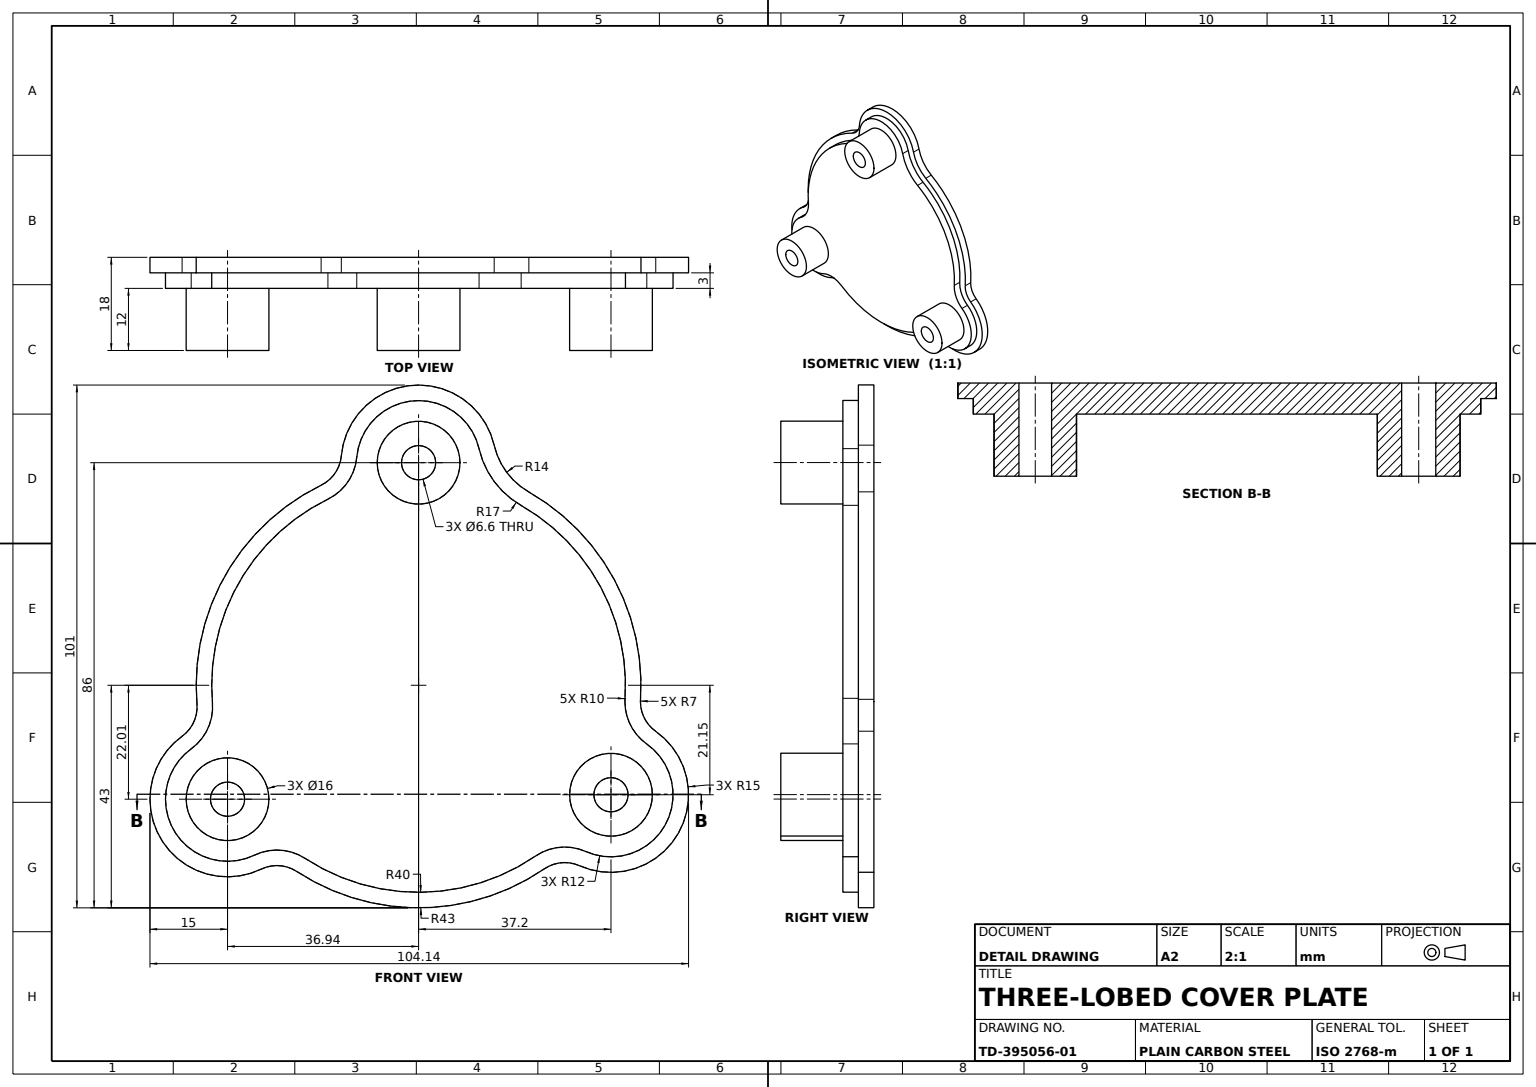
from build123d import *

# Parameters (mm, degrees)
BASE_PLATE_DEPTH               = 3
OFFSET_STEP_DEPTH              = 3
STANDOFF_BOSS_PROFILE_3X_16_R  = 8
STANDOFF_BOSSES_3X_16_DEPTH    = 12
MOUNTING_HOLE_PROFILE_3X_6_6_R = 3.3
MOUNTING_HOLES_3X_6_6_DEPTH    = 66


with BuildPart() as part:
    # Base Plate Profile → Base Plate (new body)
    with BuildSketch(Plane.XY):
        with BuildLine():
            ThreePointArc((42.912667435, -2.73915564), (37.856365651, 20.393518081), (21.320581008, 37.342105263))
            ThreePointArc((21.320581008, 37.342105263), (17.024750702, 41.150119272), (14.618361477, 46.362068966))
            ThreePointArc((14.618361477, 46.362068966), (-1.031761946, 57.964473505), (-14.941453584, 44.323995772))
            ThreePointArc((-14.941453584, 44.323995772), (-16.147655157, 40.973517523), (-18.846153454, 38.65))
            ThreePointArc((-18.846153454, 38.65), (-37.385977476, 21.243556391), (-42.849619055, -3.593069277))
            ThreePointArc((-42.849619055, -3.593069277), (-43.464441702, -7.100578343), (-45.725338247, -9.851755099))
            ThreePointArc((-45.725338247, -9.851755099), (-49.826116824, -29.687675595), (-30.429578698, -35.523293437))
            ThreePointArc((-30.429578698, -35.523293437), (-26.93387798, -34.844542215), (-23.556567678, -35.9734363))
            ThreePointArc((-23.556567678, -35.9734363), (0.447275802, -42.997673709), (24.299804013, -35.47561874))
            ThreePointArc((24.299804013, -35.47561874), (27.620379782, -34.279599541), (31.102436465, -34.855764987))
            ThreePointArc((31.102436465, -34.855764987), (50.242522242, -28.566226035), (45.85893495, -8.901909464))
            ThreePointArc((45.85893495, -8.901909464), (43.583057713, -6.204305311), (42.912667435, -2.73915564))
        make_face()
    extrude(amount=BASE_PLATE_DEPTH)

    # Offset Step Profile → Offset Step (add)
    with BuildSketch(Plane.XY.offset(3)):
        with BuildLine():
            ThreePointArc((-17.531305538, 35.953488372), (-34.777653466, 19.761447806), (-39.860110749, -3.342390025))
            ThreePointArc((-39.860110749, -3.342390025), (-40.738428815, -8.353117262), (-43.968281023, -12.283369771))
            ThreePointArc((-43.968281023, -12.283369771), (-47.248903885, -28.152106168), (-31.731673384, -32.820600441))
            ThreePointArc((-31.731673384, -32.820600441), (-26.737815215, -31.850955839), (-21.913086212, -33.463661675))
            ThreePointArc((-21.913086212, -33.463661675), (0.416070514, -39.997836008), (22.604468849, -33.000575572))
            ThreePointArc((22.604468849, -33.000575572), (27.34814852, -31.291976717), (32.32251521, -32.11507021))
            ThreePointArc((32.32251521, -32.11507021), (47.634583832, -27.083439049), (44.127713998, -11.351985792))
            ThreePointArc((44.127713998, -11.351985792), (40.876460802, -7.498265573), (39.918760405, -2.548051758))
            ThreePointArc((39.918760405, -2.548051758), (35.215223861, 18.970714494), (19.833098612, 34.736842105))
            ThreePointArc((19.833098612, 34.736842105), (14.616733241, 39.360859116), (11.694689182, 45.689655172))
            ThreePointArc((11.694689182, 45.689655172), (-0.825409557, 54.971578804), (-11.953162867, 44.059196617))
            ThreePointArc((-11.953162867, 44.059196617), (-13.676307972, 39.272799119), (-17.531305538, 35.953488372))
        make_face()
    extrude(amount=OFFSET_STEP_DEPTH)

    # Standoff Boss Profile 3xØ16 → Standoff Bosses 3xØ16 (add)
    with BuildSketch(Plane.XY.offset(6)):
        with Locations((0, 43)):
            Circle(STANDOFF_BOSS_PROFILE_3X_16_R)
        with Locations((37.202830189, -21.152291105)):
            Circle(STANDOFF_BOSS_PROFILE_3X_16_R)
        with Locations((-36.940052128, -22.009828458)):
            Circle(STANDOFF_BOSS_PROFILE_3X_16_R)
    extrude(amount=STANDOFF_BOSSES_3X_16_DEPTH)

    # Mounting Hole Profile 3xØ6.6 → Mounting Holes 3xØ6.6 (cut)
    with BuildSketch(Plane.XY.offset(18)):
        with Locations((0, 43)):
            Circle(MOUNTING_HOLE_PROFILE_3X_6_6_R)
        with Locations((37.202830189, -21.152291105)):
            Circle(MOUNTING_HOLE_PROFILE_3X_6_6_R)
        with Locations((-36.940052128, -22.009828458)):
            Circle(MOUNTING_HOLE_PROFILE_3X_6_6_R)
    extrude(amount=-MOUNTING_HOLES_3X_6_6_DEPTH, mode=Mode.SUBTRACT)


solid = part.part
